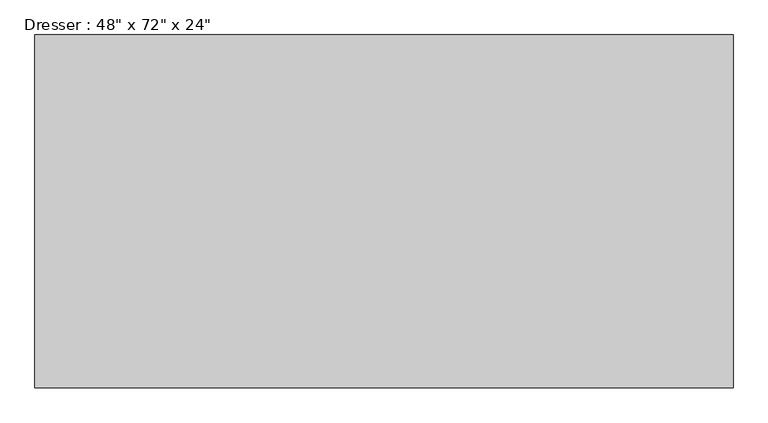
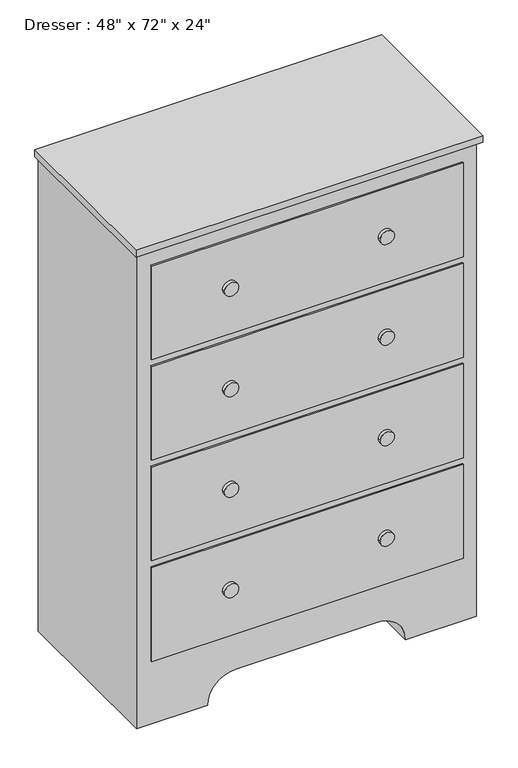
"""IFC4 building model written with IfcOpenShell, lengths in millimetres: furniture geometry."""

from ifc_helpers import new_model, si_unit, point, frame, frame_2d, origin, place, context, project, spatial, polyline, circle_curve, trimmed, segment, composite_curve, outline, extrude, source, transform, mapped, element, save


def furniture_9fa109b2(model_context):
    return source(origin(), model_context, "Body", "SweptSolid", [
        extrude(outline(polyline([(353.1067402, -58.3629541), (353.1067402, -687.0129541), (-891.4932598, -687.0129541), (-891.4932598, -58.3629541), (353.1067402, -58.3629541)])), frame((0.0, 0.0, 1803.4), z_axis=(0.0, 0.0, 1.0), x_axis=(1.0, 0.0, 0.0)), (0.0, 0.0, 1.0), 25.4),
        extrude(outline(composite_curve([segment(polyline([(0.0, 340.4067402), (1803.4, 340.4067402), (1803.4, -878.7932598), (0.0, -878.7932598), (0.0, -624.7932598)]), True, "CONTINUOUS"), segment(trimmed(circle_curve(frame_2d((0.0, -523.1932598)), 101.6), [point((0.0, -624.7932598))], [point((101.6, -523.1932598))], True, "CARTESIAN"), True, "CONTINUOUS"), segment(polyline([(101.6, -523.1932598), (101.6, -15.1932598)]), True, "CONTINUOUS"), segment(trimmed(circle_curve(frame_2d((0.0, -15.1932598)), 101.6), [point((101.6, -15.1932598))], [point((0.0, 86.4067402))], True, "CARTESIAN"), True, "CONTINUOUS"), segment(polyline([(0.0, 86.4067402), (0.0, 340.4067402)]), True, "CONTINUOUS")], self_intersect=False)), frame((0.0, -667.9629541, 0.0), z_axis=(0.0, 1.0, 0.0), x_axis=(0.0, 0.0, 1.0)), (0.0, 0.0, 1.0), 609.6),
        extrude(outline(composite_curve([segment(trimmed(circle_curve(frame_2d((1562.1, 10.2067402)), 25.4), [point((1562.1, -15.1932598))], [point((1562.1, 35.6067402))], False, "CARTESIAN"), True, "CONTINUOUS"), segment(trimmed(circle_curve(frame_2d((1562.1, 10.2067402)), 25.4), [point((1562.1, 35.6067402))], [point((1562.1, -15.1932598))], False, "CARTESIAN"), True, "CONTINUOUS")], self_intersect=False)), frame((0.0, -687.0129541, 0.0), z_axis=(0.0, 1.0, 0.0), x_axis=(0.0, 0.0, 1.0)), (0.0, 0.0, 1.0), 12.7),
        extrude(outline(composite_curve([segment(trimmed(circle_curve(frame_2d((1181.1, 10.2067402)), 25.4), [point((1181.1, -15.1932598))], [point((1181.1, 35.6067402))], False, "CARTESIAN"), True, "CONTINUOUS"), segment(trimmed(circle_curve(frame_2d((1181.1, 10.2067402)), 25.4), [point((1181.1, 35.6067402))], [point((1181.1, -15.1932598))], False, "CARTESIAN"), True, "CONTINUOUS")], self_intersect=False)), frame((0.0, -687.0129541, 0.0), z_axis=(0.0, 1.0, 0.0), x_axis=(0.0, 0.0, 1.0)), (0.0, 0.0, 1.0), 12.7),
        extrude(outline(composite_curve([segment(trimmed(circle_curve(frame_2d((800.1, 10.2067402)), 25.4), [point((800.1, -15.1932598))], [point((800.1, 35.6067402))], False, "CARTESIAN"), True, "CONTINUOUS"), segment(trimmed(circle_curve(frame_2d((800.1, 10.2067402)), 25.4), [point((800.1, 35.6067402))], [point((800.1, -15.1932598))], False, "CARTESIAN"), True, "CONTINUOUS")], self_intersect=False)), frame((0.0, -687.0129541, 0.0), z_axis=(0.0, 1.0, 0.0), x_axis=(0.0, 0.0, 1.0)), (0.0, 0.0, 1.0), 12.7),
        extrude(outline(composite_curve([segment(trimmed(circle_curve(frame_2d((419.1, 10.2067402)), 25.4), [point((419.1, -15.1932598))], [point((419.1, 35.6067402))], False, "CARTESIAN"), True, "CONTINUOUS"), segment(trimmed(circle_curve(frame_2d((419.1, 10.2067402)), 25.4), [point((419.1, 35.6067402))], [point((419.1, -15.1932598))], False, "CARTESIAN"), True, "CONTINUOUS")], self_intersect=False)), frame((0.0, -687.0129541, 0.0), z_axis=(0.0, 1.0, 0.0), x_axis=(0.0, 0.0, 1.0)), (0.0, 0.0, 1.0), 12.7),
        extrude(outline(composite_curve([segment(trimmed(circle_curve(frame_2d((419.1, -548.5932598)), 25.4), [point((419.1, -573.9932598))], [point((419.1, -523.1932598))], False, "CARTESIAN"), True, "CONTINUOUS"), segment(trimmed(circle_curve(frame_2d((419.1, -548.5932598)), 25.4), [point((419.1, -523.1932598))], [point((419.1, -573.9932598))], False, "CARTESIAN"), True, "CONTINUOUS")], self_intersect=False)), frame((0.0, -687.0129541, 0.0), z_axis=(0.0, 1.0, 0.0), x_axis=(0.0, 0.0, 1.0)), (0.0, 0.0, 1.0), 12.7),
        extrude(outline(composite_curve([segment(trimmed(circle_curve(frame_2d((800.1, -548.5932598)), 25.4), [point((800.1, -573.9932598))], [point((800.1, -523.1932598))], False, "CARTESIAN"), True, "CONTINUOUS"), segment(trimmed(circle_curve(frame_2d((800.1, -548.5932598)), 25.4), [point((800.1, -523.1932598))], [point((800.1, -573.9932598))], False, "CARTESIAN"), True, "CONTINUOUS")], self_intersect=False)), frame((0.0, -687.0129541, 0.0), z_axis=(0.0, 1.0, 0.0), x_axis=(0.0, 0.0, 1.0)), (0.0, 0.0, 1.0), 12.7),
        extrude(outline(composite_curve([segment(trimmed(circle_curve(frame_2d((1181.1, -548.5932598)), 25.4), [point((1181.1, -573.9932598))], [point((1181.1, -523.1932598))], False, "CARTESIAN"), True, "CONTINUOUS"), segment(trimmed(circle_curve(frame_2d((1181.1, -548.5932598)), 25.4), [point((1181.1, -523.1932598))], [point((1181.1, -573.9932598))], False, "CARTESIAN"), True, "CONTINUOUS")], self_intersect=False)), frame((0.0, -687.0129541, 0.0), z_axis=(0.0, 1.0, 0.0), x_axis=(0.0, 0.0, 1.0)), (0.0, 0.0, 1.0), 12.7),
        extrude(outline(composite_curve([segment(trimmed(circle_curve(frame_2d((1562.1, -548.5932598)), 25.4), [point((1562.1, -573.9932598))], [point((1562.1, -523.1932598))], False, "CARTESIAN"), True, "CONTINUOUS"), segment(trimmed(circle_curve(frame_2d((1562.1, -548.5932598)), 25.4), [point((1562.1, -523.1932598))], [point((1562.1, -573.9932598))], False, "CARTESIAN"), True, "CONTINUOUS")], self_intersect=False)), frame((0.0, -687.0129541, 0.0), z_axis=(0.0, 1.0, 0.0), x_axis=(0.0, 0.0, 1.0)), (0.0, 0.0, 1.0), 12.7),
        extrude(outline(polyline([(289.6067402, -674.3129541), (-827.9932598, -674.3129541), (-827.9932598, -667.9629541), (289.6067402, -667.9629541), (289.6067402, -674.3129541)])), frame((0.0, 0.0, 1384.3), z_axis=(0.0, 0.0, 1.0), x_axis=(1.0, 0.0, 0.0)), (0.0, 0.0, 1.0), 355.6),
        extrude(outline(polyline([(289.6067402, -674.3129541), (-827.9932598, -674.3129541), (-827.9932598, -667.9629541), (289.6067402, -667.9629541), (289.6067402, -674.3129541)])), frame((0.0, 0.0, 1003.3), z_axis=(0.0, 0.0, 1.0), x_axis=(1.0, 0.0, 0.0)), (0.0, 0.0, 1.0), 355.6),
        extrude(outline(polyline([(289.6067402, -674.3129541), (-827.9932598, -674.3129541), (-827.9932598, -667.9629541), (289.6067402, -667.9629541), (289.6067402, -674.3129541)])), frame((0.0, 0.0, 622.3), z_axis=(0.0, 0.0, 1.0), x_axis=(1.0, 0.0, 0.0)), (0.0, 0.0, 1.0), 355.6),
        extrude(outline(polyline([(289.6067402, -674.3129541), (-827.9932598, -674.3129541), (-827.9932598, -667.9629541), (289.6067402, -667.9629541), (289.6067402, -674.3129541)])), frame((0.0, 0.0, 241.3), z_axis=(0.0, 0.0, 1.0), x_axis=(1.0, 0.0, 0.0)), (0.0, 0.0, 1.0), 355.6),
    ])


if __name__ == "__main__":
    model = new_model("IFC4")
    model_context = context("Model", 3, world=origin())
    ifc_project = project(units=[si_unit("LENGTHUNIT", "METRE", prefix="MILLI")], contexts=[model_context])
    site = spatial("IfcSite", under=ifc_project)
    building = spatial("IfcBuilding", under=site)
    placement = place(None, origin())
    furniture_shape = furniture_9fa109b2(model_context)
    element("IfcFurniture", 1, ObjectType="Dresser : 48\" x 72\" x 24\"", at=placement, inside=building, context=model_context, shape_type="MappedRepresentation", body=[
        mapped(furniture_shape, transform((0.0, 0.0, 0.0), x_axis=(1.0, 0.0, 0.0), y_axis=(0.0, 1.0, 0.0), z_axis=(0.0, 0.0, 1.0))),
    ])
    save(model, "model.ifc")

# Revit data of these elements
# Type "Dresser : 48\" x 72\" x 24\""
#   Assembly Code = "E2020200"
#   Depth = 2' - 0"
#   Height = 6' - 0"
#   Width = 4' - 0"
#   Dresser Material = Wood Door Panel - Birch
#   Drawer Material = Wood Door Panel - Birch
#   Knob Material = Cherry
#   Default Elevation = 0
# Element 1 (IfcFurniture, "Dresser : 48\" x 72\" x 24\"")
#   Materials on its faces: "Laminate, Ivory, Matte", "Cherry", "Wood Door Panel - Birch"
# Materials
#   "Wood Door Panel - Birch": class "Wood", colour RGB 166 116 52, transparency 0
#   "Cherry": class "Wood", colour RGB 226 177 128, transparency 0, Description = "Prunus Serotina", Cost = 0
#   "Laminate, Ivory, Matte": class "Plastic", colour RGB 247 247 239, transparency 0, Description = "Plastic Laminate - Ivory, Matte", Cost = 0
